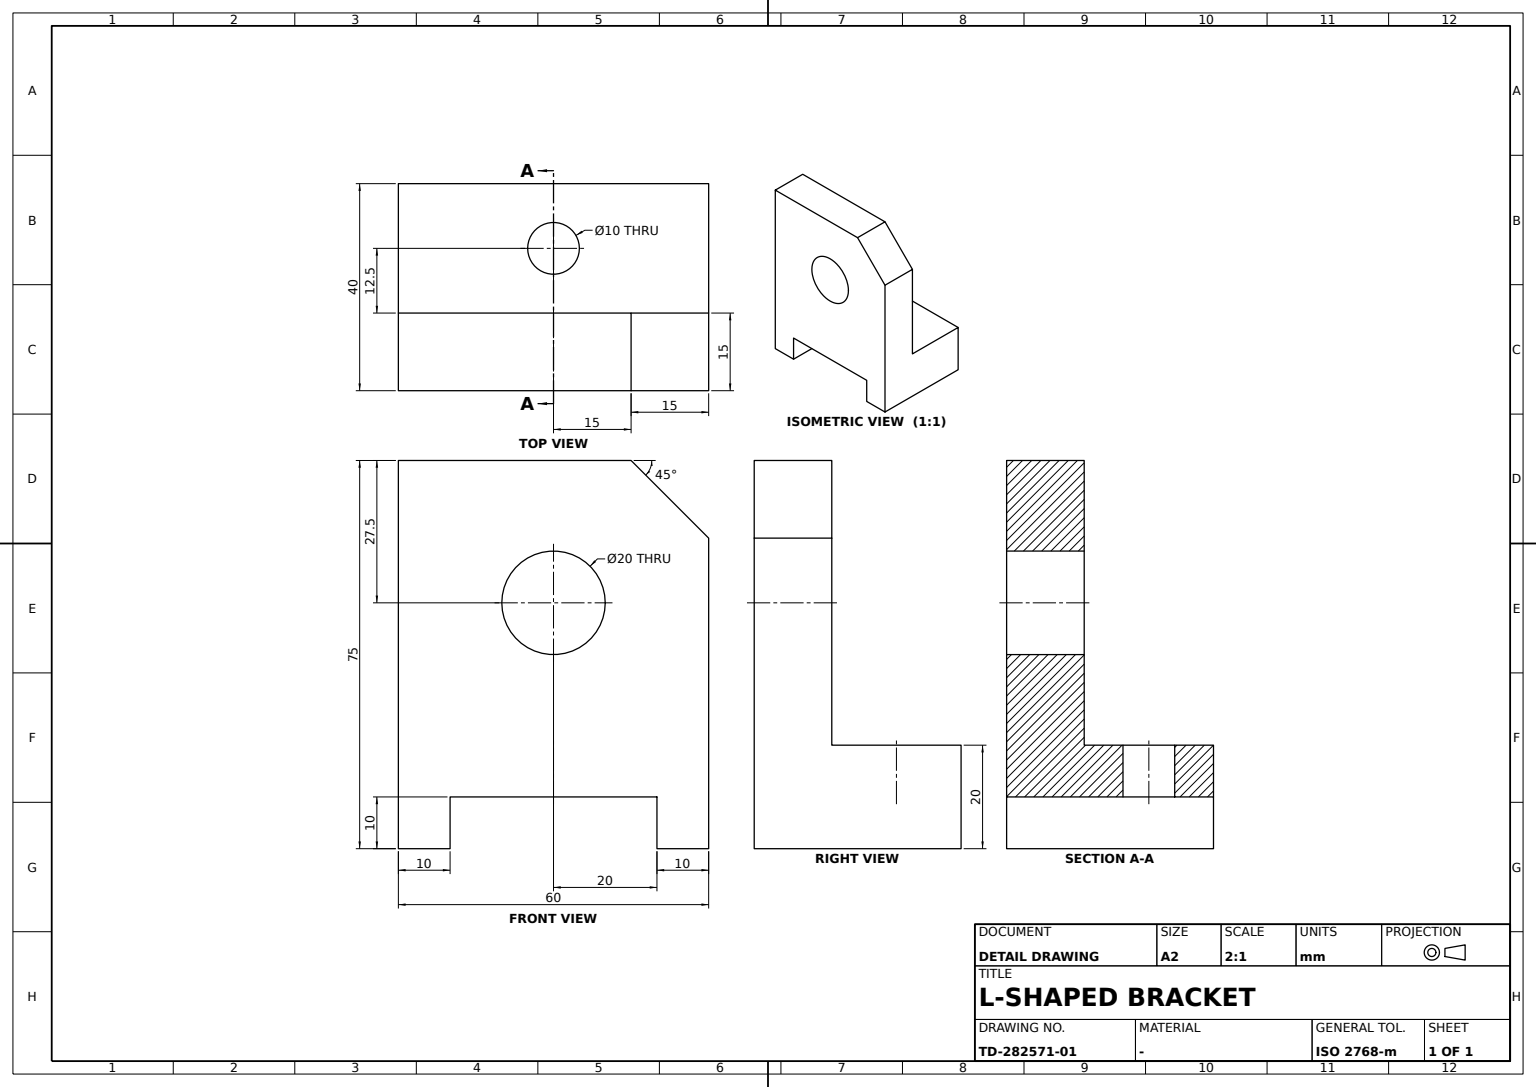
CATIA V5 part; units mm, degrees
sketch "Sketch1" plane through (0, 0, 0) normal (1, 0, 0) x (0, 1, 0)
  line L0 (-20, 0) -> (20, 0)
  line L1 (-20, 0) -> (-20, 75)
  line L2 (20, 0) -> (20, 20)
  line L3 (20, 20) -> (-5, 20)
  line L4 (-5, 20) -> (-5, 75)
  line L5 (-5, 75) -> (-20, 75)
  dimension "length L0" = 40
  dimension "length L1" = 75
  dimension "length L2" = 20
  dimension "length L3" = 25
  constraint midpoint L0 origin
  constraint horizontal L0 x-axis
  constraint horizontal L3 x-axis
  constraint horizontal L5 x-axis
  constraint vertical L1 y-axis
  constraint vertical L2 y-axis
  constraint vertical L4 y-axis
extrude "Pad1" add sketch "Sketch1" along normal mid plane 60
chamfer "Chamfer1" distance 15 distance2 15 1 edges at (30, -12.5, 75)
sketch "Sketch2" plane through (0, -5, 0) normal (0, 1, 0) x (-1, 0, 0)
  circle A0 centre (0, 47.5) radius 10
  point P0 (0, 47.5)
  line L0 (30, 75) -> (-30, 75) construction
  dimension "radius A0" = 10
  dimension "distance P0 L0" = 27.5
  constraint coincidence P0 y-axis
extrude "Pocket1" cut sketch "Sketch2" against normal up to next
sketch "Sketch3" plane through (0, 0, 20) normal (0, 0, 1) x (-1, 0, 0)
  circle A0 centre (0, -7.5) radius 5
  point P0 (0, -7.5)
  line L0 (30, -20) -> (-30, -20) construction
  dimension "radius A0" = 5
  dimension "distance P0 L0" = 12.5
  constraint coincidence P0 y-axis
extrude "Pocket2" cut sketch "Sketch3" against normal up to next
sketch "Sketch4" plane through (0, 20, 0) normal (0, 1, 0) x (-1, 0, 0)
  line L0 (-20, 0) -> (20, 0)
  line L1 (30, 0) -> (-30, 0) construction
  line L2 (-20, 0) -> (-20, 10)
  line L3 (-20, 10) -> (20, 10)
  line L4 (20, 10) -> (20, 0)
  dimension "length L0" = 40
  dimension "distance L3 L0" = 10
  constraint midpoint L0 origin
  constraint horizontal L0 x-axis
  constraint horizontal L3 x-axis
  constraint coincidence L0 L1
  constraint vertical L2 y-axis
  constraint vertical L4 y-axis
extrude "Pocket3" cut sketch "Sketch4" against normal through all
properties part number "L-Shaped Bracket with Chamfered Corner and Mounting Holes"
